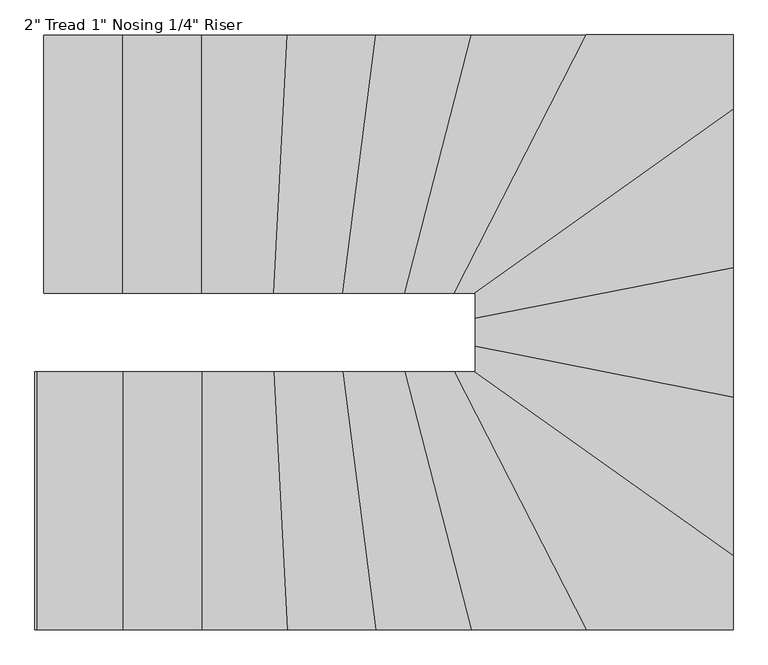
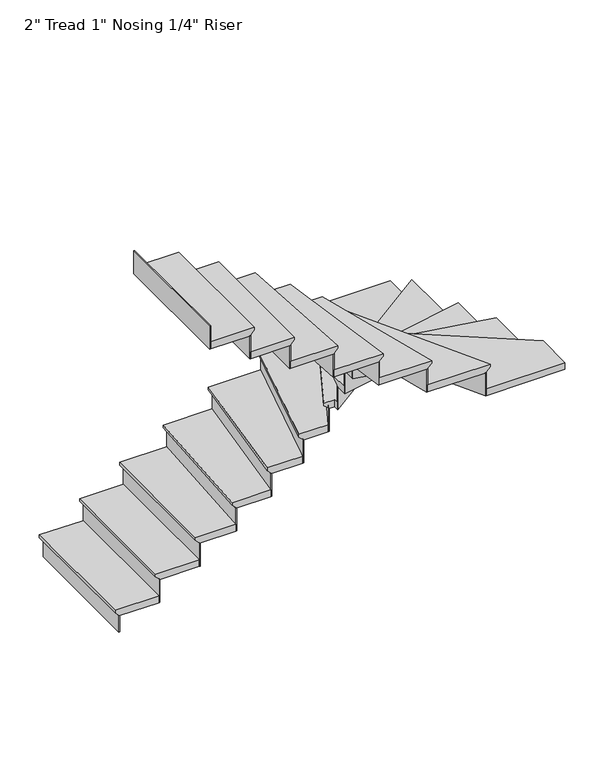
"""IFC4 building model written with IfcOpenShell, lengths in millimetres: stair flight geometry."""

from ifc_helpers import new_model, si_unit, origin, place, context, project, spatial, faceted_brep, source, transform, mapped, element, save


def stair_flight_9cd34823(model_context):
    return source(origin(), model_context, "Body", "Brep", [
        faceted_brep([(-10015.5903884, 4213.4085318, 150.2833333), (-10015.5903884, 4213.4085318, 169.3333333), (-10015.5903884, 5127.8085318, 169.3333333), (-10015.5903884, 5127.8085318, 150.2833333), (-9990.1903884, 4213.4085318, 124.8833333), (-9990.1903884, 5127.8085318, 124.8833333), (-9710.7903884, 4213.4085318, 169.3333333), (-9710.7903884, 5127.8085318, 169.3333333), (-9990.1903884, 5127.8085318, 118.5333333), (-9710.7903884, 5127.8085318, 118.5333333), (-9710.7903884, 4213.4085318, 118.5333333), (-9990.1903884, 4213.4085318, 118.5333333)], [[[0, 1, 2, 3]], [[4, 0, 3, 5]], [[2, 1, 6, 7]], [[8, 9, 10, 11]], [[2, 7, 9, 8, 5, 3]], [[8, 11, 4, 5]], [[6, 1, 0, 4, 11, 10]], [[7, 6, 10, 9]]]),
        faceted_brep([(-9990.1903884, 4213.4085318, 118.5333333), (-9990.1903884, 4213.4085318, 0.0), (-9983.8403884, 4213.4085318, 0.0), (-9983.8403884, 4213.4085318, 118.5333333), (-9990.1903884, 5127.8085318, 118.5333333), (-9983.8403884, 5127.8085318, 118.5333333), (-9983.8403884, 5127.8085318, 0.0), (-9990.1903884, 5127.8085318, 0.0)], [[[0, 1, 2, 3]], [[4, 5, 6, 7]], [[1, 0, 4, 7]], [[2, 1, 7, 6]], [[3, 2, 6, 5]], [[0, 3, 5, 4]]]),
        faceted_brep([(-9710.7903884, 4213.4085318, 287.8666667), (-9710.7903884, 4213.4085318, 118.5333333), (-9704.4403884, 4213.4085318, 118.5333333), (-9704.4403884, 4213.4085318, 287.8666667), (-9710.7903884, 5127.8085318, 287.8666667), (-9704.4403884, 5127.8085318, 287.8666667), (-9704.4403884, 5127.8085318, 118.5333333), (-9710.7903884, 5127.8085318, 118.5333333)], [[[0, 1, 2, 3]], [[4, 5, 6, 7]], [[1, 0, 4, 7]], [[2, 1, 7, 6]], [[3, 2, 6, 5]], [[0, 3, 5, 4]]]),
        faceted_brep([(-9736.1903884, 5127.8085318, 338.6666667), (-9736.1903884, 4213.4085318, 338.6666667), (-9431.3903884, 4213.4085318, 338.6666667), (-9431.3903884, 5127.8085318, 338.6666667), (-9710.7903884, 5127.8085318, 287.8666667), (-9431.3903884, 5127.8085318, 287.8666667), (-9431.3903884, 4213.4085318, 287.8666667), (-9710.7903884, 4213.4085318, 287.8666667), (-9710.7903884, 5127.8085318, 294.2166667), (-9736.1903884, 5127.8085318, 319.6166667), (-9710.7903884, 4213.4085318, 294.2166667), (-9736.1903884, 4213.4085318, 319.6166667)], [[[0, 1, 2, 3]], [[4, 5, 6, 7]], [[0, 3, 5, 4, 8, 9]], [[4, 7, 10, 8]], [[2, 1, 11, 10, 7, 6]], [[3, 2, 6, 5]], [[11, 1, 0, 9]], [[10, 11, 9, 8]]]),
        faceted_brep([(-9431.3903884, 4213.4085318, 457.2), (-9431.3903884, 4213.4085318, 287.8666667), (-9425.0403884, 4213.4085318, 287.8666667), (-9425.0403884, 4213.4085318, 457.2), (-9431.3903884, 5127.8085318, 457.2), (-9425.0403884, 5127.8085318, 457.2), (-9425.0403884, 5127.8085318, 287.8666667), (-9431.3903884, 5127.8085318, 287.8666667)], [[[0, 1, 2, 3]], [[4, 5, 6, 7]], [[1, 0, 4, 7]], [[2, 1, 7, 6]], [[3, 2, 6, 5]], [[0, 3, 5, 4]]]),
        faceted_brep([(-9456.7903884, 5127.8085318, 508.0), (-9456.7903884, 4213.4085318, 508.0), (-9175.723227, 4213.4085318, 508.0), (-9128.1889565, 5127.8085318, 508.0), (-9431.3903884, 5127.8085318, 457.2), (-9128.1889565, 5127.8085318, 457.2), (-9175.723227, 4213.4085318, 457.2), (-9431.3903884, 4213.4085318, 457.2), (-9431.3903884, 5127.8085318, 463.55), (-9456.7903884, 5127.8085318, 488.95), (-9431.3903884, 4213.4085318, 463.55), (-9456.7903884, 4213.4085318, 488.95)], [[[0, 1, 2, 3]], [[4, 5, 6, 7]], [[0, 3, 5, 4, 8, 9]], [[4, 7, 10, 8]], [[2, 1, 11, 10, 7, 6]], [[3, 2, 6, 5]], [[11, 1, 0, 9]], [[10, 11, 9, 8]]]),
        faceted_brep([(-9175.723227, 4213.4085318, 626.5333333), (-9175.723227, 4213.4085318, 457.2), (-9169.3646528, 4213.4085318, 457.2), (-9169.3646528, 4213.4085318, 626.5333333), (-9128.1889565, 5127.8085318, 626.5333333), (-9121.8303824, 5127.8085318, 626.5333333), (-9121.8303824, 5127.8085318, 457.2), (-9128.1889565, 5127.8085318, 457.2)], [[[0, 1, 2, 3]], [[4, 5, 6, 7]], [[1, 0, 4, 7]], [[2, 1, 7, 6]], [[3, 2, 6, 5]], [[0, 3, 5, 4]]]),
        faceted_brep([(-9153.6232532, 5127.8085318, 677.3333333), (-9201.1575236, 4213.4085318, 677.3333333), (-8931.5565271, 4213.4085318, 677.3333333), (-8813.2004755, 5127.8085318, 677.3333333), (-9128.1889565, 5127.8085318, 626.5333333), (-8813.2004755, 5127.8085318, 626.5333333), (-8931.5565271, 4213.4085318, 626.5333333), (-9175.723227, 4213.4085318, 626.5333333), (-9128.1889565, 5127.8085318, 632.8833333), (-9153.6232532, 5127.8085318, 658.2833333), (-9175.723227, 4213.4085318, 632.8833333), (-9201.1575236, 4213.4085318, 658.2833333)], [[[0, 1, 2, 3]], [[4, 5, 6, 7]], [[0, 3, 5, 4, 8, 9]], [[4, 7, 10, 8]], [[2, 1, 11, 10, 7, 6]], [[3, 2, 6, 5]], [[11, 1, 0, 9]], [[10, 11, 9, 8]]]),
        faceted_brep([(-8931.5565271, 4213.4085318, 795.8666667), (-8931.5565271, 4213.4085318, 626.5333333), (-8925.1535553, 4213.4085318, 626.5333333), (-8925.1535553, 4213.4085318, 795.8666667), (-8813.2004755, 5127.8085318, 795.8666667), (-8806.7975037, 5127.8085318, 795.8666667), (-8806.7975037, 5127.8085318, 626.5333333), (-8813.2004755, 5127.8085318, 626.5333333)], [[[0, 1, 2, 3]], [[4, 5, 6, 7]], [[1, 0, 4, 7]], [[2, 1, 7, 6]], [[3, 2, 6, 5]], [[0, 3, 5, 4]]]),
        faceted_brep([(-8838.8123626, 5127.8085318, 846.6666667), (-8957.1684142, 4213.4085318, 846.6666667), (-8709.9293047, 4213.4085318, 846.6666667), (-8474.7988572, 5127.8085318, 846.6666667), (-8813.2004755, 5127.8085318, 795.8666667), (-8474.7988572, 5127.8085318, 795.8666667), (-8709.9293047, 4213.4085318, 795.8666667), (-8931.5565271, 4213.4085318, 795.8666667), (-8813.2004755, 5127.8085318, 802.2166667), (-8838.8123626, 5127.8085318, 827.6166667), (-8931.5565271, 4213.4085318, 802.2166667), (-8957.1684142, 4213.4085318, 827.6166667)], [[[0, 1, 2, 3]], [[4, 5, 6, 7]], [[0, 3, 5, 4, 8, 9]], [[4, 7, 10, 8]], [[2, 1, 11, 10, 7, 6]], [[3, 2, 6, 5]], [[11, 1, 0, 9]], [[10, 11, 9, 8]]]),
        faceted_brep([(-8709.9293047, 4213.4085318, 965.2), (-8709.9293047, 4213.4085318, 795.8666667), (-8703.3727278, 4213.4085318, 795.8666667), (-8703.3727278, 4213.4085318, 965.2), (-8474.7988572, 5127.8085318, 965.2), (-8468.2422804, 5127.8085318, 965.2), (-8468.2422804, 5127.8085318, 795.8666667), (-8474.7988572, 5127.8085318, 795.8666667)], [[[0, 1, 2, 3]], [[4, 5, 6, 7]], [[1, 0, 4, 7]], [[2, 1, 7, 6]], [[3, 2, 6, 5]], [[0, 3, 5, 4]]]),
        faceted_brep([(-8501.0251647, 5127.8085318, 1016.0), (-8736.1556121, 4213.4085318, 1016.0), (-8533.5826686, 4213.4085318, 1016.0), (-8064.7580472, 5127.8085318, 1016.0), (-8474.7988572, 5127.8085318, 965.2), (-8064.7580472, 5127.8085318, 965.2), (-8533.5826686, 4213.4085318, 965.2), (-8709.9293047, 4213.4085318, 965.2), (-8474.7988572, 5127.8085318, 971.55), (-8501.0251647, 5127.8085318, 996.95), (-8709.9293047, 4213.4085318, 971.55), (-8736.1556121, 4213.4085318, 996.95)], [[[0, 1, 2, 3]], [[4, 5, 6, 7]], [[0, 3, 5, 4, 8, 9]], [[4, 7, 10, 8]], [[2, 1, 11, 10, 7, 6]], [[3, 2, 6, 5]], [[11, 1, 0, 9]], [[10, 11, 9, 8]]]),
        faceted_brep([(-8533.5826686, 4213.4085318, 1134.5333333), (-8533.5826686, 4213.4085318, 965.2), (-8526.4466854, 4213.4085318, 965.2), (-8526.4466854, 4213.4085318, 1134.5333333), (-8064.7580472, 5127.8085318, 1134.5333333), (-8057.6220641, 5127.8085318, 1134.5333333), (-8057.6220641, 5127.8085318, 965.2), (-8064.7580472, 5127.8085318, 965.2)], [[[0, 1, 2, 3]], [[4, 5, 6, 7]], [[1, 0, 4, 7]], [[2, 1, 7, 6]], [[3, 2, 6, 5]], [[0, 3, 5, 4]]]),
        faceted_brep([(-7573.4586966, 4834.1273981, 1185.3333333), (-7573.4586966, 5127.8085318, 1185.3333333), (-8093.3019798, 5127.8085318, 1185.3333333), (-8562.1266011, 4213.4085318, 1185.3333333), (-8487.8586966, 4213.4085318, 1185.3333333), (-8487.8586966, 4183.8534489, 1185.3333333), (-7573.4586966, 5127.8085318, 1134.5333333), (-7573.4586966, 4834.1273981, 1134.5333333), (-8487.8586966, 4183.8534489, 1134.5333333), (-8487.8586966, 4213.4085318, 1134.5333333), (-8533.5826686, 4213.4085318, 1134.5333333), (-8064.7580472, 5127.8085318, 1134.5333333), (-8064.7580472, 5127.8085318, 1140.8833333), (-8093.3019798, 5127.8085318, 1166.2833333), (-8533.5826686, 4213.4085318, 1140.8833333), (-8562.1266011, 4213.4085318, 1166.2833333)], [[[0, 1, 2, 3, 4, 5]], [[6, 7, 8, 9, 10, 11]], [[1, 0, 7, 6]], [[2, 1, 6, 11, 12, 13]], [[11, 10, 14, 12]], [[4, 3, 15, 14, 10, 9]], [[5, 4, 9, 8]], [[0, 5, 8, 7]], [[15, 3, 2, 13]], [[14, 15, 13, 12]]]),
        faceted_brep([(-8487.8586966, 4183.8534489, 1303.8666667), (-8487.8586966, 4183.8534489, 1134.5333333), (-8487.8586966, 4176.0614741, 1134.5333333), (-8487.8586966, 4176.0614741, 1303.8666667), (-7573.4586966, 4834.1273981, 1303.8666667), (-7573.4586966, 4826.3354233, 1303.8666667), (-7573.4586966, 4826.3354233, 1134.5333333), (-7573.4586966, 4834.1273981, 1134.5333333)], [[[0, 1, 2, 3]], [[4, 5, 6, 7]], [[1, 0, 4, 7]], [[2, 1, 7, 6]], [[3, 2, 6, 5]], [[0, 3, 5, 4]]]),
        faceted_brep([(-7573.4586966, 4865.2952972, 1354.6666667), (-8487.8586966, 4215.0213481, 1354.6666667), (-8487.8586966, 4097.3993618, 1354.6666667), (-7573.4586966, 4277.6402182, 1354.6666667), (-7573.4586966, 4834.1273981, 1303.8666667), (-7573.4586966, 4277.6402182, 1303.8666667), (-8487.8586966, 4097.3993618, 1303.8666667), (-8487.8586966, 4183.8534489, 1303.8666667), (-7573.4586966, 4834.1273981, 1310.2166667), (-7573.4586966, 4865.2952972, 1335.6166667), (-8487.8586966, 4183.8534489, 1310.2166667), (-8487.8586966, 4215.0213481, 1335.6166667)], [[[0, 1, 2, 3]], [[4, 5, 6, 7]], [[0, 3, 5, 4, 8, 9]], [[4, 7, 10, 8]], [[2, 1, 11, 10, 7, 6]], [[3, 2, 6, 5]], [[11, 1, 0, 9]], [[10, 11, 9, 8]]]),
        faceted_brep([(-8487.8586966, 4097.3993618, 1473.2), (-8487.8586966, 4097.3993618, 1303.8666667), (-8487.8586966, 4090.9271764, 1303.8666667), (-8487.8586966, 4090.9271764, 1473.2), (-7573.4586966, 4277.6402182, 1473.2), (-7573.4586966, 4271.1680327, 1473.2), (-7573.4586966, 4271.1680327, 1303.8666667), (-7573.4586966, 4277.6402182, 1303.8666667)], [[[0, 1, 2, 3]], [[4, 5, 6, 7]], [[1, 0, 4, 7]], [[2, 1, 7, 6]], [[3, 2, 6, 5]], [[0, 3, 5, 4]]]),
        faceted_brep([(-7573.4586966, 4303.5289599, 1524.0), (-8487.8586966, 4123.2881036, 1524.0), (-8487.8586966, 3998.2402182, 1524.0), (-7573.4586966, 3817.9993618, 1524.0), (-7573.4586966, 4277.6402182, 1473.2), (-7573.4586966, 3817.9993618, 1473.2), (-8487.8586966, 3998.2402182, 1473.2), (-8487.8586966, 4097.3993618, 1473.2), (-7573.4586966, 4277.6402182, 1479.55), (-7573.4586966, 4303.5289599, 1504.95), (-8487.8586966, 4097.3993618, 1479.55), (-8487.8586966, 4123.2881036, 1504.95)], [[[0, 1, 2, 3]], [[4, 5, 6, 7]], [[0, 3, 5, 4, 8, 9]], [[4, 7, 10, 8]], [[2, 1, 11, 10, 7, 6]], [[3, 2, 6, 5]], [[11, 1, 0, 9]], [[10, 11, 9, 8]]]),
        faceted_brep([(-8487.8586966, 3998.2402182, 1642.5333333), (-8487.8586966, 3998.2402182, 1473.2), (-8487.8586966, 3991.7680327, 1473.2), (-8487.8586966, 3991.7680327, 1642.5333333), (-7573.4586966, 3817.9993618, 1642.5333333), (-7573.4586966, 3811.5271764, 1642.5333333), (-7573.4586966, 3811.5271764, 1473.2), (-7573.4586966, 3817.9993618, 1473.2)], [[[0, 1, 2, 3]], [[4, 5, 6, 7]], [[1, 0, 4, 7]], [[2, 1, 7, 6]], [[3, 2, 6, 5]], [[0, 3, 5, 4]]]),
        faceted_brep([(-7573.4586966, 3843.8881036, 1693.3333333), (-8487.8586966, 4024.1289599, 1693.3333333), (-8487.8586966, 3934.0085318, 1693.3333333), (-8533.9541711, 3934.0085318, 1693.3333333), (-7573.4586966, 3250.9538671, 1693.3333333), (-7573.4586966, 3817.9993618, 1642.5333333), (-7573.4586966, 3250.9538671, 1642.5333333), (-8533.9541711, 3934.0085318, 1642.5333333), (-8487.8586966, 3934.0085318, 1642.5333333), (-8487.8586966, 3998.2402182, 1642.5333333), (-7573.4586966, 3817.9993618, 1648.8833333), (-7573.4586966, 3843.8881036, 1674.2833333), (-8487.8586966, 3998.2402182, 1648.8833333), (-8487.8586966, 4024.1289599, 1674.2833333)], [[[0, 1, 2, 3, 4]], [[5, 6, 7, 8, 9]], [[0, 4, 6, 5, 10, 11]], [[5, 9, 12, 10]], [[2, 1, 13, 12, 9, 8]], [[3, 2, 8, 7]], [[4, 3, 7, 6]], [[13, 1, 0, 11]], [[12, 13, 11, 10]]]),
        faceted_brep([(-8533.9541711, 3934.0085318, 1811.8666667), (-8533.9541711, 3934.0085318, 1642.5333333), (-8544.9110636, 3934.0085318, 1642.5333333), (-8544.9110636, 3934.0085318, 1811.8666667), (-7573.4586966, 3250.9538671, 1811.8666667), (-7573.4586966, 3243.1618923, 1811.8666667), (-7573.4586966, 3243.1618923, 1642.5333333), (-7573.4586966, 3250.9538671, 1642.5333333)], [[[0, 1, 2, 3]], [[4, 5, 6, 7]], [[1, 0, 4, 7]], [[2, 1, 7, 6]], [[3, 2, 6, 5]], [[0, 3, 5, 4]]]),
        faceted_brep([(-8121.8459123, 3019.6085318, 1862.6666667), (-7573.4586966, 3019.6085318, 1862.6666667), (-7573.4586966, 3282.1217663, 1862.6666667), (-8490.1266011, 3934.0085318, 1862.6666667), (-8590.6705336, 3934.0085318, 1862.6666667), (-7573.4586966, 3019.6085318, 1811.8666667), (-8121.8459123, 3019.6085318, 1811.8666667), (-8590.6705336, 3934.0085318, 1811.8666667), (-8533.9541711, 3934.0085318, 1811.8666667), (-7573.4586966, 3250.9538671, 1811.8666667), (-7573.4586966, 3250.9538671, 1818.2166667), (-7573.4586966, 3282.1217663, 1843.6166667), (-8533.9541711, 3934.0085318, 1818.2166667), (-8490.1266011, 3934.0085318, 1843.6166667)], [[[0, 1, 2, 3, 4]], [[5, 6, 7, 8, 9]], [[1, 0, 6, 5]], [[2, 1, 5, 9, 10, 11]], [[9, 8, 12, 10]], [[4, 3, 13, 12, 8, 7]], [[0, 4, 7, 6]], [[13, 3, 2, 11]], [[12, 13, 11, 10]]]),
        faceted_brep([(-8590.6705336, 3934.0085318, 1981.2), (-8590.6705336, 3934.0085318, 1811.8666667), (-8597.8065168, 3934.0085318, 1811.8666667), (-8597.8065168, 3934.0085318, 1981.2), (-8121.8459123, 3019.6085318, 1981.2), (-8128.9818954, 3019.6085318, 1981.2), (-8128.9818954, 3019.6085318, 1811.8666667), (-8121.8459123, 3019.6085318, 1811.8666667)], [[[0, 1, 2, 3]], [[4, 5, 6, 7]], [[1, 0, 4, 7]], [[2, 1, 7, 6]], [[3, 2, 6, 5]], [[0, 3, 5, 4]]]),
        faceted_brep([(-8093.3019798, 3019.6085318, 2032.0), (-8562.1266011, 3934.0085318, 2032.0), (-8762.3819196, 3934.0085318, 2032.0), (-8527.2514722, 3019.6085318, 2032.0), (-8121.8459123, 3019.6085318, 1981.2), (-8527.2514722, 3019.6085318, 1981.2), (-8762.3819196, 3934.0085318, 1981.2), (-8590.6705336, 3934.0085318, 1981.2), (-8121.8459123, 3019.6085318, 1987.55), (-8093.3019798, 3019.6085318, 2012.95), (-8590.6705336, 3934.0085318, 1987.55), (-8562.1266011, 3934.0085318, 2012.95)], [[[0, 1, 2, 3]], [[4, 5, 6, 7]], [[0, 3, 5, 4, 8, 9]], [[4, 7, 10, 8]], [[2, 1, 11, 10, 7, 6]], [[3, 2, 6, 5]], [[11, 1, 0, 9]], [[10, 11, 9, 8]]]),
        faceted_brep([(-8762.3819196, 3934.0085318, 2150.5333333), (-8762.3819196, 3934.0085318, 1981.2), (-8768.9384964, 3934.0085318, 1981.2), (-8768.9384964, 3934.0085318, 2150.5333333), (-8527.2514722, 3019.6085318, 2150.5333333), (-8533.808049, 3019.6085318, 2150.5333333), (-8533.808049, 3019.6085318, 1981.2), (-8527.2514722, 3019.6085318, 1981.2)], [[[0, 1, 2, 3]], [[4, 5, 6, 7]], [[1, 0, 4, 7]], [[2, 1, 7, 6]], [[3, 2, 6, 5]], [[0, 3, 5, 4]]]),
        faceted_brep([(-8501.0251647, 3019.6085318, 2201.3333333), (-8736.1556121, 3934.0085318, 2201.3333333), (-8982.7803014, 3934.0085318, 2201.3333333), (-8864.4242497, 3019.6085318, 2201.3333333), (-8527.2514722, 3019.6085318, 2150.5333333), (-8864.4242497, 3019.6085318, 2150.5333333), (-8982.7803014, 3934.0085318, 2150.5333333), (-8762.3819196, 3934.0085318, 2150.5333333), (-8527.2514722, 3019.6085318, 2156.8833333), (-8501.0251647, 3019.6085318, 2182.2833333), (-8762.3819196, 3934.0085318, 2156.8833333), (-8736.1556121, 3934.0085318, 2182.2833333)], [[[0, 1, 2, 3]], [[4, 5, 6, 7]], [[0, 3, 5, 4, 8, 9]], [[4, 7, 10, 8]], [[2, 1, 11, 10, 7, 6]], [[3, 2, 6, 5]], [[11, 1, 0, 9]], [[10, 11, 9, 8]]]),
        faceted_brep([(-8982.7803014, 3934.0085318, 2319.8666667), (-8982.7803014, 3934.0085318, 2150.5333333), (-8989.1832731, 3934.0085318, 2150.5333333), (-8989.1832731, 3934.0085318, 2319.8666667), (-8864.4242497, 3019.6085318, 2319.8666667), (-8870.8272215, 3019.6085318, 2319.8666667), (-8870.8272215, 3019.6085318, 2150.5333333), (-8864.4242497, 3019.6085318, 2150.5333333)], [[[0, 1, 2, 3]], [[4, 5, 6, 7]], [[1, 0, 4, 7]], [[2, 1, 7, 6]], [[3, 2, 6, 5]], [[0, 3, 5, 4]]]),
        faceted_brep([(-8838.8123626, 3019.6085318, 2370.6666667), (-8957.1684142, 3934.0085318, 2370.6666667), (-9226.5918203, 3934.0085318, 2370.6666667), (-9179.0575499, 3019.6085318, 2370.6666667), (-8864.4242497, 3019.6085318, 2319.8666667), (-9179.0575499, 3019.6085318, 2319.8666667), (-9226.5918203, 3934.0085318, 2319.8666667), (-8982.7803014, 3934.0085318, 2319.8666667), (-8864.4242497, 3019.6085318, 2326.2166667), (-8838.8123626, 3019.6085318, 2351.6166667), (-8982.7803014, 3934.0085318, 2326.2166667), (-8957.1684142, 3934.0085318, 2351.6166667)], [[[0, 1, 2, 3]], [[4, 5, 6, 7]], [[0, 3, 5, 4, 8, 9]], [[4, 7, 10, 8]], [[2, 1, 11, 10, 7, 6]], [[3, 2, 6, 5]], [[11, 1, 0, 9]], [[10, 11, 9, 8]]]),
        faceted_brep([(-9226.5918203, 3934.0085318, 2489.2), (-9226.5918203, 3934.0085318, 2319.8666667), (-9232.9503944, 3934.0085318, 2319.8666667), (-9232.9503944, 3934.0085318, 2489.2), (-9179.0575499, 3019.6085318, 2489.2), (-9185.416124, 3019.6085318, 2489.2), (-9185.416124, 3019.6085318, 2319.8666667), (-9179.0575499, 3019.6085318, 2319.8666667)], [[[0, 1, 2, 3]], [[4, 5, 6, 7]], [[1, 0, 4, 7]], [[2, 1, 7, 6]], [[3, 2, 6, 5]], [[0, 3, 5, 4]]]),
        faceted_brep([(-9153.6232532, 3019.6085318, 2540.0), (-9201.1575236, 3934.0085318, 2540.0), (-9482.1903884, 3934.0085318, 2540.0), (-9482.1903884, 3019.6085318, 2540.0), (-9179.0575499, 3019.6085318, 2489.2), (-9482.1903884, 3019.6085318, 2489.2), (-9482.1903884, 3934.0085318, 2489.2), (-9226.5918203, 3934.0085318, 2489.2), (-9179.0575499, 3019.6085318, 2495.55), (-9153.6232532, 3019.6085318, 2520.95), (-9226.5918203, 3934.0085318, 2495.55), (-9201.1575236, 3934.0085318, 2520.95)], [[[0, 1, 2, 3]], [[4, 5, 6, 7]], [[0, 3, 5, 4, 8, 9]], [[4, 7, 10, 8]], [[2, 1, 11, 10, 7, 6]], [[3, 2, 6, 5]], [[11, 1, 0, 9]], [[10, 11, 9, 8]]]),
        faceted_brep([(-9482.1903884, 3934.0085318, 2658.5333333), (-9482.1903884, 3934.0085318, 2489.2), (-9488.5403884, 3934.0085318, 2489.2), (-9488.5403884, 3934.0085318, 2658.5333333), (-9482.1903884, 3019.6085318, 2658.5333333), (-9488.5403884, 3019.6085318, 2658.5333333), (-9488.5403884, 3019.6085318, 2489.2), (-9482.1903884, 3019.6085318, 2489.2)], [[[0, 1, 2, 3]], [[4, 5, 6, 7]], [[1, 0, 4, 7]], [[2, 1, 7, 6]], [[3, 2, 6, 5]], [[0, 3, 5, 4]]]),
        faceted_brep([(-9456.7903884, 3019.6085318, 2709.3333333), (-9456.7903884, 3934.0085318, 2709.3333333), (-9761.5903884, 3934.0085318, 2709.3333333), (-9761.5903884, 3019.6085318, 2709.3333333), (-9482.1903884, 3019.6085318, 2658.5333333), (-9761.5903884, 3019.6085318, 2658.5333333), (-9761.5903884, 3934.0085318, 2658.5333333), (-9482.1903884, 3934.0085318, 2658.5333333), (-9482.1903884, 3019.6085318, 2664.8833333), (-9456.7903884, 3019.6085318, 2690.2833333), (-9482.1903884, 3934.0085318, 2664.8833333), (-9456.7903884, 3934.0085318, 2690.2833333)], [[[0, 1, 2, 3]], [[4, 5, 6, 7]], [[0, 3, 5, 4, 8, 9]], [[4, 7, 10, 8]], [[2, 1, 11, 10, 7, 6]], [[3, 2, 6, 5]], [[11, 1, 0, 9]], [[10, 11, 9, 8]]]),
        faceted_brep([(-9761.5903884, 3934.0085318, 2827.8666667), (-9761.5903884, 3934.0085318, 2658.5333333), (-9767.9403884, 3934.0085318, 2658.5333333), (-9767.9403884, 3934.0085318, 2827.8666667), (-9761.5903884, 3019.6085318, 2827.8666667), (-9767.9403884, 3019.6085318, 2827.8666667), (-9767.9403884, 3019.6085318, 2658.5333333), (-9761.5903884, 3019.6085318, 2658.5333333)], [[[0, 1, 2, 3]], [[4, 5, 6, 7]], [[1, 0, 4, 7]], [[2, 1, 7, 6]], [[3, 2, 6, 5]], [[0, 3, 5, 4]]]),
        faceted_brep([(-10040.9903884, 3934.0085318, 2997.2), (-10040.9903884, 3934.0085318, 2827.8666667), (-10047.3403884, 3934.0085318, 2827.8666667), (-10047.3403884, 3934.0085318, 2997.2), (-10040.9903884, 3019.6085318, 2997.2), (-10047.3403884, 3019.6085318, 2997.2), (-10047.3403884, 3019.6085318, 2827.8666667), (-10040.9903884, 3019.6085318, 2827.8666667)], [[[0, 1, 2, 3]], [[4, 5, 6, 7]], [[1, 0, 4, 7]], [[2, 1, 7, 6]], [[3, 2, 6, 5]], [[0, 3, 5, 4]]]),
        faceted_brep([(-9736.1903884, 3019.6085318, 2878.6666667), (-9736.1903884, 3934.0085318, 2878.6666667), (-10040.9903884, 3934.0085318, 2878.6666667), (-10040.9903884, 3019.6085318, 2878.6666667), (-9761.5903884, 3019.6085318, 2827.8666667), (-10040.9903884, 3019.6085318, 2827.8666667), (-10040.9903884, 3934.0085318, 2827.8666667), (-9761.5903884, 3934.0085318, 2827.8666667), (-9761.5903884, 3019.6085318, 2834.2166667), (-9736.1903884, 3019.6085318, 2859.6166667), (-9761.5903884, 3934.0085318, 2834.2166667), (-9736.1903884, 3934.0085318, 2859.6166667)], [[[0, 1, 2, 3]], [[4, 5, 6, 7]], [[0, 3, 5, 4, 8, 9]], [[4, 7, 10, 8]], [[2, 1, 11, 10, 7, 6]], [[3, 2, 6, 5]], [[11, 1, 0, 9]], [[10, 11, 9, 8]]]),
    ])


if __name__ == "__main__":
    model = new_model("IFC4")
    model_context = context("Model", 3, world=origin())
    ifc_project = project(units=[si_unit("LENGTHUNIT", "METRE", prefix="MILLI")], contexts=[model_context])
    site = spatial("IfcSite", under=ifc_project)
    building = spatial("IfcBuilding", under=site)
    placement = place(None, origin())
    stair_flight_shape = stair_flight_9cd34823(model_context)
    element("IfcStairFlight", 1, ObjectType="2\" Tread 1\" Nosing 1/4\" Riser", at=placement, inside=building, context=model_context, shape_type="MappedRepresentation", body=[
        mapped(stair_flight_shape, transform((0.0, 0.0, 0.0), x_axis=(1.0, 0.0, 0.0), y_axis=(0.0, 1.0, 0.0), z_axis=(0.0, 0.0, 1.0))),
    ])
    save(model, "model.ifc")
